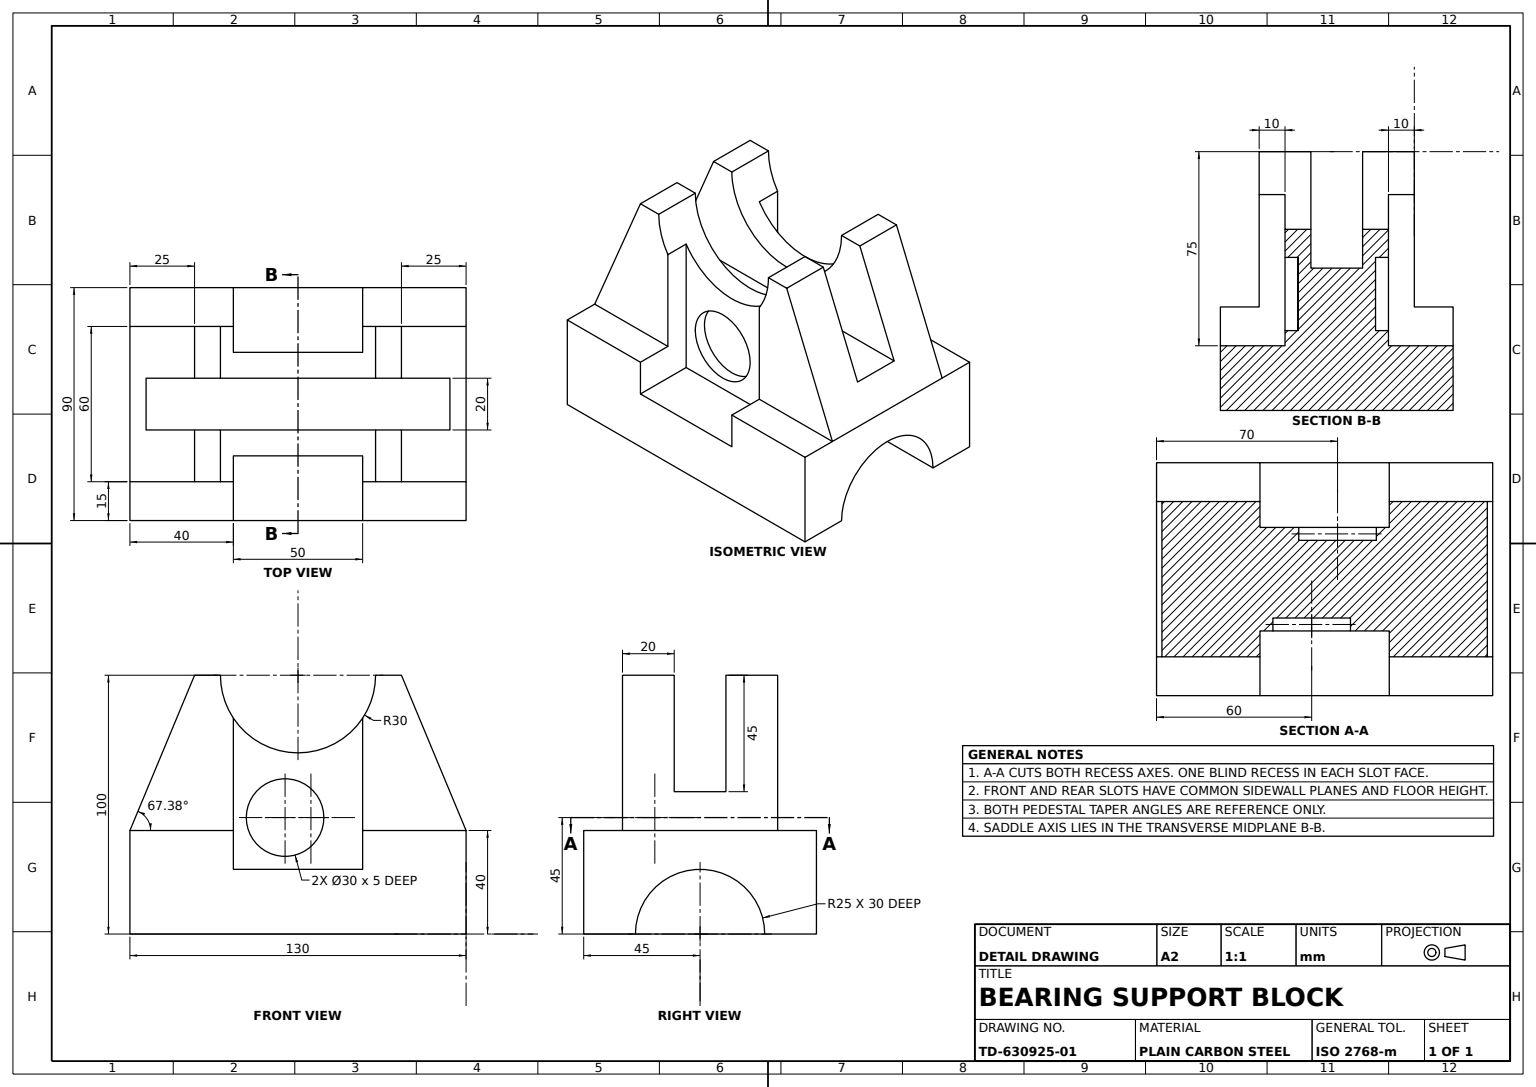
SolidWorks part; units mm, degrees
material "Plain Carbon Steel"
ref_plane "Front Plane" through (0, 0, 0) normal (0, 0, 1) x (1, 0, 0)
ref_plane "Top Plane" through (0, 0, 0) normal (0, 1, 0) x (1, 0, 0)
ref_plane "Right Plane" through (0, 0, 0) normal (1, 0, 0) x (0, 0, -1)
sketch "Base Block Profile" plane through (0, 0, 0) normal (0, 0, 1) x (1, 0, 0)
  line L0 (0, 0) -> (25, 0)
  line L1 (25, 0) -> (25, 15)
  line L2 (25, 15) -> (65, 15)
  line L3 (65, 15) -> (65, -25)
  line L4 (65, -25) -> (-65, -25)
  line L5 (-65, -25) -> (-65, 15)
  line L6 (-65, 15) -> (-25, 15)
  line L7 (-25, 15) -> (-25, 0)
  line L8 (-25, 0) -> (0, 0)
  dimension "D1" = 25
  dimension "D2" = 130
  dimension "D3" = 40
  dimension "D4" = 40
  dimension "D5" = 40
  dimension "D6" = 25
extrude "Base Block" add sketch "Base Block Profile" along normal mid plane 90
sketch "Bottom Arch Profile R25" plane through (65, 0, 0) normal (1, 0, 0) x (0, 0, -1)
  line L0 (-45, -25) -> (45, -25) construction
  line L1 (-25, -25) -> (25, -25)
  arc A0 (25, -25) -> (-25, -25) centre (0, -25) ccw
  dimension "D1" = 25
extrude "Bottom Arch Cut" cut sketch "Bottom Arch Profile R25" against normal blind 30
sketch "Pedestal Profile" plane through (0, 0, 45) normal (0, 0, 1) x (1, 0, 0)
  line L0 (-65, 15) -> (-40, 75)
  line L1 (-40, 75) -> (40, 75)
  line L2 (40, 75) -> (65, 15)
  line L3 (0, 0) -> (0, 75) construction
  line L4 (-65, 15) -> (-25, 15)
  line L5 (-25, 15) -> (-25, 0)
  line L6 (-25, 0) -> (25, 0)
  line L7 (25, 0) -> (25, 15)
  line L8 (25, 15) -> (65, 15)
  dimension "D1" = 40
  dimension "D2" = 40
  dimension "D3" = 60
extrude "Bearing Pedestal" add sketch "Pedestal Profile" against normal blind 75
sketch "Pedestal Side Cut Profile" plane through (0, 0, 45) normal (0, 0, 1) x (1, 0, 0)
  line L0 (-65, 15) -> (-25, 15)
  line L1 (-25, 15) -> (-25, 0)
  line L2 (-25, 0) -> (25, 0)
  line L3 (25, 0) -> (25, 15)
  line L4 (25, 15) -> (65, 15)
  line L5 (65, 15) -> (40, 75)
  line L6 (40, 75) -> (-40, 75)
  line L7 (-40, 75) -> (-65, 15)
  line L8 (-65, 15) -> (-65, -25) construction
  line L9 (-65, -25) -> (65, -25) construction
  dimension "D1" = 40
  dimension "D2" = 25
extrude "Pedestal Side Cut" cut sketch "Pedestal Side Cut Profile" against normal blind 15
sketch "Bearing Seat Profile" plane through (0, 75, 0) normal (0, 1, 0) x (1, 0, 0)
  line L0 (65, -30) -> (65, 30) construction
  line L1 (-65, 10) -> (65, 10)
  line L2 (-65, 10) -> (-65, -10)
  line L3 (-65, -10) -> (65, -10)
  line L4 (65, 10) -> (65, -10)
  line L5 (-65, 10) -> (65, -10) construction
  line L6 (-65, -10) -> (65, 10) construction
  point P0 (0, 0)
  dimension "D1" = 20
extrude "Bearing Seat Cut" cut sketch "Bearing Seat Profile" against normal blind 45
sketch "Cross Hole Profile" plane through (0, 0, 10) normal (0, 0, -1) x (-1, 0, 0)
  line L0 (40, 75) -> (-40, 75) construction
  line L1 (-30, 75) -> (30, 75)
  arc A0 (-30, 75) -> (30, 75) centre (0, 75) ccw
  dimension "D1" = 30
extrude "Cross Hole" cut sketch "Cross Hole Profile" against normal through all both and the other way through all
sketch "Slot A Profile" plane through (0, 0, 30) normal (0, 0, 1) x (1, 0, 0)
  line L0 (-25, 0) -> (-25, 58.4169)
  line L1 (-25, 0) -> (25, 0)
  line L2 (25, 0) -> (25, 58.4169)
  arc A0 (-30, 75) -> (30, 75) centre (0, 75) ccw construction
  arc A1 (-25, 58.4169) -> (25, 58.4169) centre (0, 75) ccw
extrude "Slot A Cut" cut sketch "Slot A Profile" against normal blind 10
sketch "Slot B Profile" plane through (0, 0, -30) normal (0, 0, -1) x (-1, 0, 0)
  line L0 (-25, 0) -> (25, 0)
  line L1 (25, 0) -> (25, 58.4169)
  line L2 (-25, 0) -> (-25, 58.4169)
  arc A0 (-30, 75) -> (30, 75) centre (0, 75) ccw construction
  arc A1 (-25, 58.4169) -> (25, 58.4169) centre (0, 75) ccw
extrude "Slot B Cut" cut sketch "Slot B Profile" against normal blind 10
sketch "Step Recess A Profile" plane through (0, 0, -20) normal (0, 0, -1) x (-1, 0, 0)
  line L0 (-25, 0) -> (-5, 0) construction
  line L1 (-25, 0) -> (25, 0) construction
  line L2 (-5, 0) -> (-5, 20) construction
  circle A0 centre (-5, 20) radius 15
  dimension "D1" = 30
  dimension "D2" = 20
  dimension "D3" = 20
extrude "Step Recess A" cut sketch "Step Recess A Profile" against normal blind 5
sketch "Step Recess B Profile" plane through (0, 0, 20) normal (0, 0, 1) x (1, 0, 0)
  line L0 (-25, 0) -> (-5, 0) construction
  line L1 (-25, 0) -> (25, 0) construction
  line L2 (-5, 0) -> (-5, 20) construction
  circle A0 centre (-5, 20) radius 15
  dimension "D1" = 30
  dimension "D2" = 20
  dimension "D3" = 20
extrude "Step Recess B" cut sketch "Step Recess B Profile" against normal blind 5
